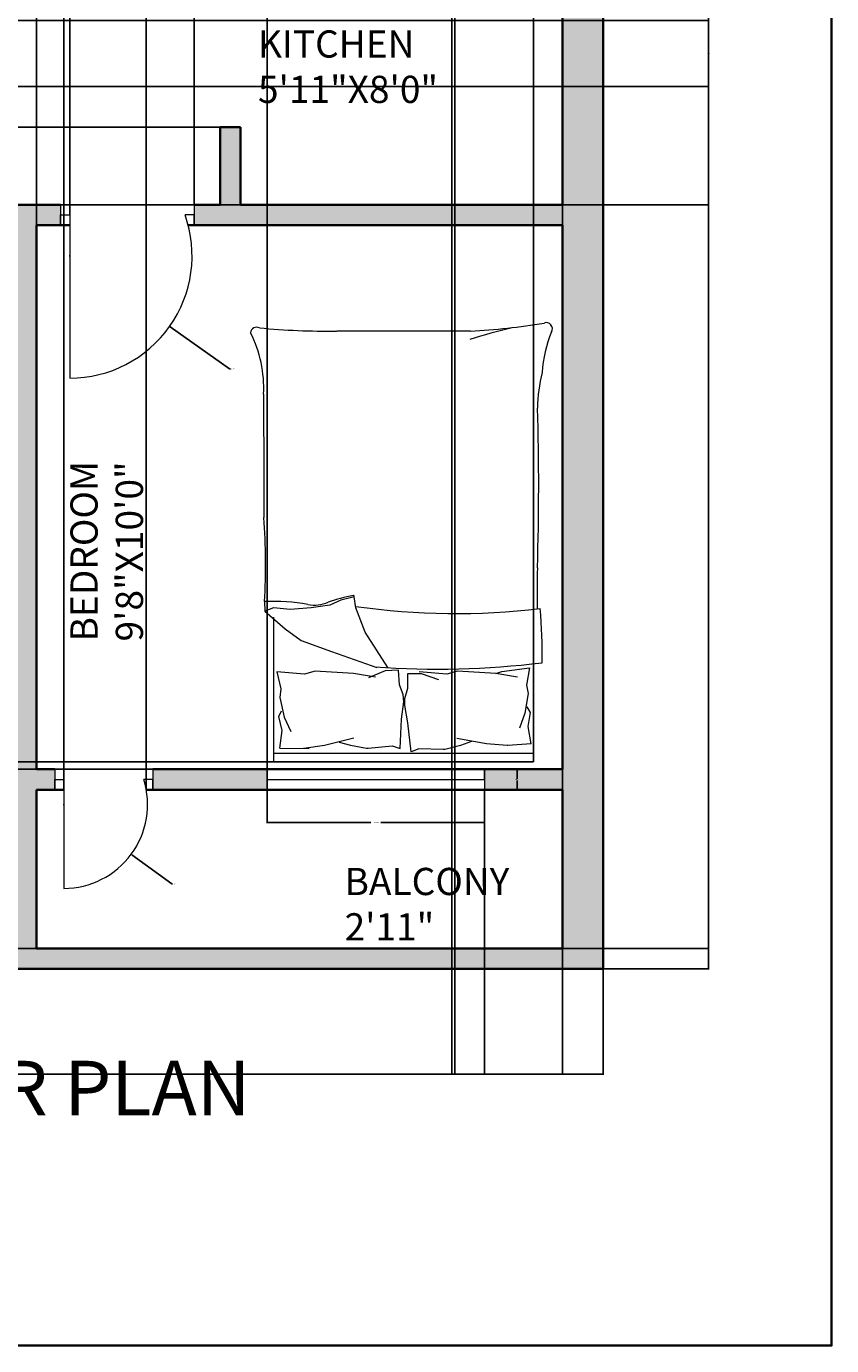
# Model space of a CAD drawing. Units: inches. Extents: x 2606 to 3027, y 1906 to 2463.
# Tile 4 of 10: x 2850 to 3027, y 1906 to 2196. Entities that reach past the tile are written whole.
import ezdxf

# ---------------------------------------------------------------- set-up
doc = ezdxf.new("R2010")
doc.units = ezdxf.units.IN
for name, color, linetype, lineweight in [('A-ANNO-DIMS', 2, 'Continuous', 18), ('A-ANNO-TEXT', 7, 'Continuous', 25), ('A-ANNO-TTLB', 7, 'Continuous', 35), ('A-AREA-IDEN', 7, 'Continuous', 18), ('A-DOOR', 3, 'Continuous', 18), ('A-FLOR-CASE', 8, 'Continuous', 18), ('A-FURN', 8, 'Continuous', 13), ('A-GLAZ', 4, 'Continuous', 18), ('A-WALL', 7, 'Continuous', 35)]:
    doc.layers.add(name, color=color, linetype=linetype, lineweight=lineweight)
doc.layers.add('A-WALL-PATT', color=251, linetype='Continuous', lineweight=13, true_color=0x636466)
doc.styles.get("Standard").update_dxf_attribs({"font": 'arial.ttf'})
doc.dimstyles.get("Standard").update_dxf_attribs({"dimtxt": 0.18, "dimasz": 0.18, "dimexe": 0.18, "dimexo": 0.0625, "dimgap": 0.09, "dimtad": 0, "dimtih": 1, "dimtoh": 1, "dimdec": 4, "dimzin": 0, "dimdsep": 46, "dimtxsty": 'Standard', "dimcen": 0.09, "dimadec": 0, "dimazin": 0, "dimtfac": 1, "dimtdec": 4, "dimtofl": 0, "dimtmove": 0, "dimatfit": 3, "dimfxl": 1, "dimtolj": 1, "dimtzin": 0, "dimarcsym": 0})

# ---------------------------------------------------------------- blocks, each defined once
blk = doc.blocks.new('BED-DOUBLE')
for p, q in [((4.17, 75.16), (4.17, 96.87)), ((4.17, 96.87), (61.46, 96.87)), ((61.46, 96.87), (61.46, 64.97)), ((4.17, 95.03), (61.46, 95.03)), ((4.67, 92.87), (9.81, 93.27)), ((9.81, 93.27), (9.93, 93.24)), ((9.93, 93.24), (14.52, 92.9)), ((17.81, 92.38), (20.24, 93.24)), ((20.24, 93.24), (23.7, 94.11)), ((23.7, 94.11), (24.09, 94.11)), ((24.09, 94.11), (29.42, 93.94)), ((29.42, 93.94), (31.15, 94.63)), ((31.15, 94.63), (31.84, 88.22)), ((33.54, 93.89), (33.25, 87.44)), ((35.31, 93.3), (33.54, 93.89)), ((40.62, 93.81), (35.31, 93.3)), ((41.01, 93.83), (40.62, 93.81)), ((44.52, 93.18), (41.01, 93.83)), ((50.25, 93.19), (43.75, 91.57)), ((47, 92.47), (44.52, 93.18)), ((54.8, 93.82), (50.25, 93.19)), ((60.08, 93.81), (53.6, 93.92)), ((53.6, 93.92), (54.8, 93.82)), ((60.08, 93.81), (59.62, 89.96)), ((4.67, 92.9), (5.36, 89.08)), ((14.52, 92.9), (21.1, 91.68)), ((59.12, 86.97), (57.7, 90.18)), ((5.36, 89.08), (4.84, 85.96)), ((6.06, 86.14), (7.27, 89.43)), ((31.84, 88.22), (32.54, 84.4)), ((33.25, 87.44), (32.79, 83.59)), ((59.62, 89.96), (60.34, 86.88)), ((4.84, 85.96), (5.54, 84.75)), ((5.36, 81.8), (6.06, 86.14)), ((32.54, 84.4), (32.54, 82.84)), ((60.08, 82.69), (59.12, 86.97)), ((60.34, 86.88), (59.72, 85.62)), ((5.71, 79.9), (5.36, 81.8)), ((32.54, 82.84), (31.84, 80.59)), ((32.79, 83.59), (32.89, 82.03)), ((32.89, 82.03), (33.72, 79.83)), ((59.85, 80.77), (60.08, 82.69)), ((5.02, 76.08), (5.71, 79.9)), ((28.9, 77.38), (25.13, 78.68)), ((31.84, 80.59), (31.84, 77.38)), ((33.72, 79.83), (33.92, 76.62)), ((60.78, 77), (59.85, 80.77)), ((11.13, 76.95), (5.02, 76.08)), ((7.65, 78.14), (12.48, 77.34)), ((12.48, 77.34), (11.13, 76.95)), ((12.48, 77.34), (20.89, 76.82)), ((20.89, 76.82), (23.24, 77.49)), ((23.24, 77.49), (29.39, 77)), ((31.84, 77.38), (28.9, 77.38)), ((33.92, 76.62), (36.87, 76.8)), ((36.28, 76.03), (41.3, 68.25)), ((36.87, 76.8), (40.55, 78.34)), ((48.73, 72.52), (38.73, 76.03)), ((39.04, 78.14), (43.87, 77.34)), ((43.87, 77.34), (52.28, 76.82)), ((52.28, 76.82), (54.63, 77.49)), ((54.63, 77.49), (60.78, 77)), ((55.41, 70.1), (48.73, 72.52)), ((58.94, 67.51), (55.41, 70.1)), ((41.3, 68.25), (43.34, 62.87)), ((63.38, 63.61), (58.94, 67.51)), ((43.34, 62.87), (43.71, 60.45)), ((43.71, 60.45), (46.68, 61.2)), ((46.68, 61.2), (49.1, 62.31)), ((49.1, 62.31), (53.18, 62.87)), ((53.18, 62.87), (57.82, 63.24)), ((57.82, 63.24), (61.54, 62.87)), ((61.54, 62.87), (63.38, 63.61)), ((63.48, 61.52), (63.38, 63.61, 4.64)), ((18.06, 1.87), (47.57, 1.87))]:
    blk.add_line(p, q)
for centre, radius, start, end in [((25.61, -121.38), 197.77, 86.0865, 96.7821), ((102.1, 72.78), 99.87, 178.7218, 185.604), ((21.29, -90.53), 154.68, 81.7845, 96.9006), ((-200.58, 59.5), 203.94, 358.4762, 1.0082), ((37.35, 95.1), 35.55, 280.6617, 289.8806), ((52.44, 54.83), 7.46, 78.6608, 113.7384), ((61.53, 104.85), 43.38, 259.8763, 272.5657), ((218.51, 53.34), 155.25, 176.9791, 183.8365), ((43.92, 60.38), 0.221, 160.2464, 271.1377), ((581.23, 36.19), 578.22, 178.22771, 181.71854), ((-5405.34, 15.56), 5469.02, 0.00217, 0.28689), ((-32.25, 19.53), 35.53, 346.0648, 358.9113), ((91.3, 14.55), 27.65, 177.4714, 206.4681), ((-25.97, 12.62), 28.25, 337.9751, 356.652), ((-20.65, 125.3), 127.63, 283.3832, 287.7053), ((1.3, 1.3), 1.31, 146.1736, 293.4781), ((25.69, -143.9), 145.97, 92.9958, 99.4091), ((49.34, -157.62), 159.5, 84.4998, 90.6351), ((65.23, 2.32), 1.32, 242.6588, 356.02)]:
    blk.add_arc(centre, radius, start, end)
blk = doc.blocks.new('WIN-48IN')
for p, q in [((0, 4.5), (0, 0)), ((48, 2.25), (48, 4.5)), ((48, 4.5), (48, 0)), ((0, 0), (0, 2.25)), ((0, 2.25), (48, 2.25))]:
    blk.add_line(p, q)
blk = doc.blocks.new('*D13')
at = {"layer": 'A-ANNO-DIMS', "color": 0, "lineweight": -2, "transparency": 16777216}
for p, q in [((2902.89, 2028.05), (2902.89, 2020.73)), ((2950.89, 2028.05), (2950.89, 2020.73)), ((2903.07, 2020.91), (2925.77, 2020.91)), ((2950.71, 2020.91), (2928.01, 2020.91))]:
    blk.add_line(p, q, dxfattribs=at)
at = {"layer": 'A-ANNO-DIMS', "color": 0, "transparency": 16777216}
for points in [[(2903.07, 2020.94), (2903.07, 2020.88), (2902.89, 2020.91)], [(2950.71, 2020.94), (2950.71, 2020.88), (2950.89, 2020.91)]]:
    blk.add_solid(points, dxfattribs=at)
at = {"layer": 'Defpoints', "color": 0, "transparency": 16777216}
for p in [(2902.89, 2028.11), (2950.89, 2028.11), (2950.89, 2020.91)]:
    blk.add_point(p, dxfattribs=at)
at = {"layer": 'A-ANNO-DIMS', "color": 0, "transparency": 16777216, "insert": (2926.89, 2020.91), "char_height": 0.18, "attachment_point": 5}
blk.add_mtext('\\A1;WINDOW 48 TYP.', dxfattribs=at)
blk = doc.blocks.new('*D14')
at = {"layer": 'A-ANNO-DIMS', "color": 0, "lineweight": -2, "transparency": 16777216}
for p, q in [((2950.95, 2032.61), (2958.27, 2032.61)), ((2958.09, 2032.43), (2958.09, 2030.54)), ((2950.95, 2028.11), (2958.27, 2028.11)), ((2958.09, 2028.29), (2958.09, 2030.18))]:
    blk.add_line(p, q, dxfattribs=at)
at = {"layer": 'A-ANNO-DIMS', "color": 0, "transparency": 16777216}
for points in [[(2958.06, 2032.43), (2958.12, 2032.43), (2958.09, 2032.61)], [(2958.06, 2028.29), (2958.12, 2028.29), (2958.09, 2028.11)]]:
    blk.add_solid(points, dxfattribs=at)
at = {"layer": 'Defpoints', "color": 0, "transparency": 16777216}
for p in [(2950.89, 2032.61), (2958.09, 2032.61), (2950.89, 2028.11)]:
    blk.add_point(p, dxfattribs=at)
at = {"layer": 'A-ANNO-DIMS', "color": 0, "transparency": 16777216, "insert": (2958.09, 2030.36), "char_height": 0.18, "attachment_point": 5}
blk.add_mtext('\\A1;5 TYP.', dxfattribs=at)
blk = doc.blocks.new('*D25')
at = {"layer": 'A-ANNO-DIMS', "color": 0, "lineweight": -2, "transparency": 16777216}
for p, q in [((2658.06, 1988.55), (2658.06, 1965.23)), ((2977.06, 1988.55), (2977.06, 1965.23)), ((2658.24, 1965.41), (2817.27, 1965.41)), ((2976.88, 1965.41), (2817.85, 1965.41))]:
    blk.add_line(p, q, dxfattribs=at)
at = {"layer": 'A-ANNO-DIMS', "color": 0, "transparency": 16777216}
for points in [[(2658.24, 1965.44), (2658.24, 1965.38), (2658.06, 1965.41)], [(2976.88, 1965.44), (2976.88, 1965.38), (2977.06, 1965.41)]]:
    blk.add_solid(points, dxfattribs=at)
at = {"layer": 'Defpoints', "color": 0, "transparency": 16777216}
for p in [(2658.06, 1988.61), (2977.06, 1988.61), (2977.06, 1965.41)]:
    blk.add_point(p, dxfattribs=at)
at = {"layer": 'A-ANNO-DIMS', "color": 0, "transparency": 16777216, "insert": (2817.56, 1965.41), "char_height": 0.18, "attachment_point": 5}
blk.add_mtext('\\A1;319', dxfattribs=at)
blk = doc.blocks.new('*D26')
at = {"layer": 'A-ANNO-DIMS', "color": 0, "lineweight": -2, "transparency": 16777216}
for p, q in [((2977.13, 2410.61), (3000.44, 2410.61)), ((3000.26, 2410.43), (3000.26, 2199.79)), ((3000.26, 1988.79), (3000.26, 2199.43)), ((2977.13, 1988.61), (3000.44, 1988.61))]:
    blk.add_line(p, q, dxfattribs=at)
at = {"layer": 'A-ANNO-DIMS', "color": 0, "transparency": 16777216}
for points in [[(3000.23, 2410.43), (3000.29, 2410.43), (3000.26, 2410.61)], [(3000.23, 1988.79), (3000.29, 1988.79), (3000.26, 1988.61)]]:
    blk.add_solid(points, dxfattribs=at)
at = {"layer": 'Defpoints', "color": 0, "transparency": 16777216}
for p in [(2977.06, 2410.61), (3000.26, 2410.61), (2977.06, 1988.61)]:
    blk.add_point(p, dxfattribs=at)
at = {"layer": 'A-ANNO-DIMS', "color": 0, "transparency": 16777216, "insert": (3000.26, 2199.61), "char_height": 0.18, "attachment_point": 5}
blk.add_mtext('\\A1;422', dxfattribs=at)
blk = doc.blocks.new('*D33')
at = {"layer": 'A-ANNO-DIMS', "color": 0, "lineweight": -2, "transparency": 16777216}
for p, q in [((2950.89, 2028.05), (2950.89, 1965.23)), ((2968.06, 2028.05), (2968.06, 1965.23)), ((2951.07, 1965.41), (2959.02, 1965.41)), ((2967.88, 1965.41), (2959.93, 1965.41))]:
    blk.add_line(p, q, dxfattribs=at)
at = {"layer": 'A-ANNO-DIMS', "color": 0, "transparency": 16777216}
for points in [[(2951.07, 1965.44), (2951.07, 1965.38), (2950.89, 1965.41)], [(2967.88, 1965.44), (2967.88, 1965.38), (2968.06, 1965.41)]]:
    blk.add_solid(points, dxfattribs=at)
at = {"layer": 'Defpoints', "color": 0, "transparency": 16777216}
for p in [(2950.89, 2028.11), (2968.06, 2028.11), (2968.06, 1965.41)]:
    blk.add_point(p, dxfattribs=at)
at = {"layer": 'A-ANNO-DIMS', "color": 0, "transparency": 16777216, "insert": (2959.48, 1965.41), "char_height": 0.18, "attachment_point": 5}
blk.add_mtext('\\A1;17.172', dxfattribs=at)
blk = doc.blocks.new('*D41')
at = {"layer": 'A-ANNO-DIMS', "color": 0, "lineweight": -2, "transparency": 16777216}
for p, q in [((2787.63, 2157.11), (3000.44, 2157.11)), ((3000.26, 2156.93), (3000.26, 2075.29)), ((3000.26, 1993.29), (3000.26, 2074.93)), ((2787.63, 1993.11), (3000.44, 1993.11))]:
    blk.add_line(p, q, dxfattribs=at)
at = {"layer": 'A-ANNO-DIMS', "color": 0, "transparency": 16777216}
for points in [[(3000.23, 2156.93), (3000.29, 2156.93), (3000.26, 2157.11)], [(3000.23, 1993.29), (3000.29, 1993.29), (3000.26, 1993.11)]]:
    blk.add_solid(points, dxfattribs=at)
at = {"layer": 'Defpoints', "color": 0, "transparency": 16777216}
for p in [(2787.56, 2157.11), (2787.56, 1993.11), (3000.26, 1993.11)]:
    blk.add_point(p, dxfattribs=at)
at = {"layer": 'A-ANNO-DIMS', "color": 0, "transparency": 16777216, "insert": (3000.26, 2075.11), "char_height": 0.18, "attachment_point": 5}
blk.add_mtext('\\A1;164', dxfattribs=at)
blk = doc.blocks.new('*D46')
at = {"layer": 'A-ANNO-DIMS', "color": 0, "lineweight": -2, "transparency": 16777216}
for p, q in [((2859.37, 2154.92), (2859.37, 2433.99)), ((2859.55, 2433.81), (2872.63, 2433.81)), ((2886.63, 2433.81), (2873.56, 2433.81)), ((2886.81, 2157.17), (2886.81, 2433.99))]:
    blk.add_line(p, q, dxfattribs=at)
at = {"layer": 'A-ANNO-DIMS', "color": 0, "transparency": 16777216}
for points in [[(2859.55, 2433.84), (2859.55, 2433.78), (2859.37, 2433.81)], [(2886.63, 2433.84), (2886.63, 2433.78), (2886.81, 2433.81)]]:
    blk.add_solid(points, dxfattribs=at)
at = {"layer": 'Defpoints', "color": 0, "transparency": 16777216}
for p in [(2886.81, 2433.81), (2886.81, 2157.11), (2859.37, 2154.86)]:
    blk.add_point(p, dxfattribs=at)
at = {"layer": 'A-ANNO-DIMS', "color": 0, "transparency": 16777216, "insert": (2873.09, 2433.81), "char_height": 0.18, "attachment_point": 5}
blk.add_mtext('\\A1;27.443', dxfattribs=at)
blk = doc.blocks.new('*D48')
at = {"layer": 'A-ANNO-DIMS', "color": 0, "lineweight": -2, "transparency": 16777216}
for p, q in [((2858.07, 2028.17), (2858.07, 2433.99)), ((2858.25, 2433.81), (2866.77, 2433.81)), ((2876.06, 2433.81), (2867.54, 2433.81)), ((2876.24, 2028.17), (2876.24, 2433.99))]:
    blk.add_line(p, q, dxfattribs=at)
at = {"layer": 'A-ANNO-DIMS', "color": 0, "transparency": 16777216}
for points in [[(2858.25, 2433.84), (2858.25, 2433.78), (2858.07, 2433.81)], [(2876.06, 2433.84), (2876.06, 2433.78), (2876.24, 2433.81)]]:
    blk.add_solid(points, dxfattribs=at)
at = {"layer": 'Defpoints', "color": 0, "transparency": 16777216}
for p in [(2876.24, 2433.81), (2858.07, 2028.11), (2876.24, 2028.11)]:
    blk.add_point(p, dxfattribs=at)
at = {"layer": 'A-ANNO-DIMS', "color": 0, "transparency": 16777216, "insert": (2867.16, 2433.81), "char_height": 0.18, "attachment_point": 5}
blk.add_mtext('\\A1;18.17', dxfattribs=at)
blk = doc.blocks.new('*D55')
at = {"layer": 'A-ANNO-DIMS', "color": 0, "lineweight": -2, "transparency": 16777216}
for p, q in [((2852.06, 2152.67), (2852.06, 2433.99)), ((2852.24, 2433.81), (2855.32, 2433.81)), ((2859.19, 2433.81), (2856.11, 2433.81)), ((2859.37, 2154.92), (2859.37, 2433.99))]:
    blk.add_line(p, q, dxfattribs=at)
at = {"layer": 'A-ANNO-DIMS', "color": 0, "transparency": 16777216}
for points in [[(2852.24, 2433.84), (2852.24, 2433.78), (2852.06, 2433.81)], [(2859.19, 2433.84), (2859.19, 2433.78), (2859.37, 2433.81)]]:
    blk.add_solid(points, dxfattribs=at)
at = {"layer": 'Defpoints', "color": 0, "transparency": 16777216}
for p in [(2859.37, 2433.81), (2859.37, 2154.86), (2852.06, 2152.61)]:
    blk.add_point(p, dxfattribs=at)
at = {"layer": 'A-ANNO-DIMS', "color": 0, "transparency": 16777216, "insert": (2855.72, 2433.81), "char_height": 0.18, "attachment_point": 5}
blk.add_mtext('\\A1;7.306', dxfattribs=at)
blk = doc.blocks.new('*D57')
at = {"layer": 'A-ANNO-DIMS', "color": 0, "lineweight": -2, "transparency": 16777216}
for p, q in [((2876.24, 2028.17), (2876.24, 2433.99)), ((2876.42, 2433.81), (2889.17, 2433.81)), ((2902.71, 2433.81), (2889.96, 2433.81)), ((2902.89, 2028.17), (2902.89, 2433.99))]:
    blk.add_line(p, q, dxfattribs=at)
at = {"layer": 'A-ANNO-DIMS', "color": 0, "transparency": 16777216}
for points in [[(2876.42, 2433.84), (2876.42, 2433.78), (2876.24, 2433.81)], [(2902.71, 2433.84), (2902.71, 2433.78), (2902.89, 2433.81)]]:
    blk.add_solid(points, dxfattribs=at)
at = {"layer": 'Defpoints', "color": 0, "transparency": 16777216}
for p in [(2902.89, 2433.81), (2876.24, 2028.11), (2902.89, 2028.11)]:
    blk.add_point(p, dxfattribs=at)
at = {"layer": 'A-ANNO-DIMS', "color": 0, "transparency": 16777216, "insert": (2889.57, 2433.81), "char_height": 0.18, "attachment_point": 5}
blk.add_mtext('\\A1;26.65', dxfattribs=at)
blk = doc.blocks.new('*D61')
at = {"layer": 'A-ANNO-DIMS', "color": 0, "lineweight": -2, "transparency": 16777216}
for p, q in [((2696.29, 2197.72), (3000.44, 2197.72)), ((3000.26, 2197.54), (3000.26, 2190.63)), ((3000.26, 2183.36), (3000.26, 2190.27)), ((2696.84, 2183.18), (3000.44, 2183.18))]:
    blk.add_line(p, q, dxfattribs=at)
at = {"layer": 'A-ANNO-DIMS', "color": 0, "transparency": 16777216}
for points in [[(3000.23, 2197.54), (3000.29, 2197.54), (3000.26, 2197.72)], [(3000.23, 2183.36), (3000.29, 2183.36), (3000.26, 2183.18)]]:
    blk.add_solid(points, dxfattribs=at)
at = {"layer": 'Defpoints', "color": 0, "transparency": 16777216}
for p in [(2696.23, 2197.72), (3000.26, 2197.72), (2696.78, 2183.18)]:
    blk.add_point(p, dxfattribs=at)
at = {"layer": 'A-ANNO-DIMS', "color": 0, "transparency": 16777216, "insert": (3000.26, 2190.45), "char_height": 0.18, "attachment_point": 5}
blk.add_mtext('\\A1;14.545', dxfattribs=at)
blk = doc.blocks.new('*D66')
at = {"layer": 'A-ANNO-DIMS', "color": 0, "lineweight": -2, "transparency": 16777216}
for p, q in [((2968.06, 2253.05), (2968.06, 1965.23)), ((2944.33, 2234.06), (2944.33, 1965.23)), ((2944.51, 1965.41), (2955.8, 1965.41)), ((2967.88, 1965.41), (2956.59, 1965.41))]:
    blk.add_line(p, q, dxfattribs=at)
at = {"layer": 'A-ANNO-DIMS', "color": 0, "transparency": 16777216}
for points in [[(2944.51, 1965.44), (2944.51, 1965.38), (2944.33, 1965.41)], [(2967.88, 1965.44), (2967.88, 1965.38), (2968.06, 1965.41)]]:
    blk.add_solid(points, dxfattribs=at)
at = {"layer": 'Defpoints', "color": 0, "transparency": 16777216}
for p in [(2968.06, 2253.11), (2944.33, 2234.12), (2968.06, 1965.41)]:
    blk.add_point(p, dxfattribs=at)
at = {"layer": 'A-ANNO-DIMS', "color": 0, "transparency": 16777216, "insert": (2956.2, 1965.41), "char_height": 0.18, "attachment_point": 5}
blk.add_mtext('\\A1;23.73', dxfattribs=at)
blk = doc.blocks.new('*D68')
at = {"layer": 'A-ANNO-DIMS', "color": 0, "lineweight": -2, "transparency": 16777216}
for p, q in [((2897, 2215.13), (2634.68, 2215.13)), ((2634.86, 2214.95), (2634.86, 2194.85)), ((2634.86, 2174.38), (2634.86, 2194.48)), ((2897, 2174.2), (2634.68, 2174.2))]:
    blk.add_line(p, q, dxfattribs=at)
at = {"layer": 'A-ANNO-DIMS', "color": 0, "transparency": 16777216}
for points in [[(2634.83, 2214.95), (2634.89, 2214.95), (2634.86, 2215.13)], [(2634.83, 2174.38), (2634.89, 2174.38), (2634.86, 2174.2)]]:
    blk.add_solid(points, dxfattribs=at)
at = {"layer": 'Defpoints', "color": 0, "transparency": 16777216}
for p in [(2897.06, 2215.13), (2634.86, 2174.2), (2897.06, 2174.2)]:
    blk.add_point(p, dxfattribs=at)
at = {"layer": 'A-ANNO-DIMS', "color": 0, "transparency": 16777216, "insert": (2634.86, 2194.66), "char_height": 0.18, "attachment_point": 5}
blk.add_mtext('\\A1;40.94', dxfattribs=at)
blk = doc.blocks.new('*D69')
at = {"layer": 'A-ANNO-DIMS', "color": 0, "lineweight": -2, "transparency": 16777216}
for p, q in [((2897, 2174.2), (2634.68, 2174.2)), ((2634.86, 2174.02), (2634.86, 2165.84)), ((2634.86, 2157.29), (2634.86, 2165.47)), ((2897, 2157.11), (2634.68, 2157.11))]:
    blk.add_line(p, q, dxfattribs=at)
at = {"layer": 'A-ANNO-DIMS', "color": 0, "transparency": 16777216}
for points in [[(2634.83, 2174.02), (2634.89, 2174.02), (2634.86, 2174.2)], [(2634.83, 2157.29), (2634.89, 2157.29), (2634.86, 2157.11)]]:
    blk.add_solid(points, dxfattribs=at)
at = {"layer": 'Defpoints', "color": 0, "transparency": 16777216}
for p in [(2897.06, 2174.2), (2634.86, 2157.11), (2897.06, 2157.11)]:
    blk.add_point(p, dxfattribs=at)
at = {"layer": 'A-ANNO-DIMS', "color": 0, "transparency": 16777216, "insert": (2634.86, 2165.65), "char_height": 0.18, "attachment_point": 5}
blk.add_mtext('\\A1;17.087', dxfattribs=at)
blk = doc.blocks.new('*D75')
at = {"layer": 'A-ANNO-DIMS', "color": 0, "lineweight": -2, "transparency": 16777216}
for p, q in [((2968.06, 2401.55), (2968.06, 1965.23)), ((2943.67, 2399.33), (2943.67, 1965.23)), ((2943.85, 1965.41), (2955.4, 1965.41)), ((2967.88, 1965.41), (2956.33, 1965.41))]:
    blk.add_line(p, q, dxfattribs=at)
at = {"layer": 'A-ANNO-DIMS', "color": 0, "transparency": 16777216}
for points in [[(2943.85, 1965.44), (2943.85, 1965.38), (2943.67, 1965.41)], [(2967.88, 1965.44), (2967.88, 1965.38), (2968.06, 1965.41)]]:
    blk.add_solid(points, dxfattribs=at)
at = {"layer": 'Defpoints', "color": 0, "transparency": 16777216}
for p in [(2968.06, 2401.61), (2943.67, 2399.4), (2968.06, 1965.41)]:
    blk.add_point(p, dxfattribs=at)
at = {"layer": 'A-ANNO-DIMS', "color": 0, "transparency": 16777216, "insert": (2955.86, 1965.41), "char_height": 0.18, "attachment_point": 5}
blk.add_mtext('\\A1;24.397', dxfattribs=at)
blk = doc.blocks.new('*D77')
at = {"layer": 'A-ANNO-DIMS', "color": 0, "lineweight": -2, "transparency": 16777216}
for p, q in [((2961.66, 2034.29), (2961.66, 2433.99)), ((2961.84, 2433.81), (2964.47, 2433.81)), ((2967.88, 2433.81), (2965.26, 2433.81)), ((2968.06, 2032.67), (2968.06, 2433.99))]:
    blk.add_line(p, q, dxfattribs=at)
at = {"layer": 'A-ANNO-DIMS', "color": 0, "transparency": 16777216}
for points in [[(2961.84, 2433.84), (2961.84, 2433.78), (2961.66, 2433.81)], [(2967.88, 2433.84), (2967.88, 2433.78), (2968.06, 2433.81)]]:
    blk.add_solid(points, dxfattribs=at)
at = {"layer": 'Defpoints', "color": 0, "transparency": 16777216}
for p in [(2968.06, 2433.81), (2961.66, 2034.23), (2968.06, 2032.61)]:
    blk.add_point(p, dxfattribs=at)
at = {"layer": 'A-ANNO-DIMS', "color": 0, "transparency": 16777216, "insert": (2964.86, 2433.81), "char_height": 0.18, "attachment_point": 5}
blk.add_mtext('\\A1;6.402', dxfattribs=at)
blk = doc.blocks.new('*D81')
at = {"layer": 'A-ANNO-DIMS', "color": 0, "lineweight": -2, "transparency": 16777216}
for p, q in [((2961.6, 2034.23), (2634.68, 2034.23)), ((2634.86, 2034.05), (2634.86, 2033.6)), ((2950.83, 2032.61), (2634.68, 2032.61)), ((2634.86, 2032.79), (2634.86, 2033.24))]:
    blk.add_line(p, q, dxfattribs=at)
at = {"layer": 'A-ANNO-DIMS', "color": 0, "transparency": 16777216}
for points in [[(2634.83, 2034.05), (2634.89, 2034.05), (2634.86, 2034.23)], [(2634.83, 2032.79), (2634.89, 2032.79), (2634.86, 2032.61)]]:
    blk.add_solid(points, dxfattribs=at)
at = {"layer": 'Defpoints', "color": 0, "transparency": 16777216}
for p in [(2961.66, 2034.23), (2634.86, 2032.61), (2950.89, 2032.61)]:
    blk.add_point(p, dxfattribs=at)
at = {"layer": 'A-ANNO-DIMS', "color": 0, "transparency": 16777216, "insert": (2634.86, 2033.42), "char_height": 0.18, "attachment_point": 5}
blk.add_mtext('\\A1;1.62', dxfattribs=at)
blk = doc.blocks.new('*D87')
at = {"layer": 'A-ANNO-DIMS', "color": 0, "lineweight": -2, "transparency": 16777216}
for p, q in [((2859.28, 2145.85), (2859.46, 2145.85)), ((2859.37, 2145.76), (2859.37, 2145.94)), ((2894.64, 2120.93), (2881.56, 2130.17)), ((2894.82, 2120.93), (2894.64, 2120.93))]:
    blk.add_line(p, q, dxfattribs=at)
at = {"layer": 'A-ANNO-DIMS', "color": 0, "transparency": 16777216}
blk.add_solid([(2881.58, 2130.19), (2881.54, 2130.14), (2881.41, 2130.27)], dxfattribs=at)
at = {"layer": 'Defpoints', "color": 0, "transparency": 16777216}
for p in [(2859.37, 2145.85), (2881.41, 2130.27)]:
    blk.add_point(p, dxfattribs=at)
at = {"layer": 'A-ANNO-DIMS', "color": 0, "transparency": 16777216, "insert": (2895.3, 2120.93), "char_height": 0.18, "attachment_point": 5}
blk.add_mtext('\\A1;R26.99', dxfattribs=at)
blk = doc.blocks.new('*D89')
at = {"layer": 'A-ANNO-DIMS', "color": 0, "lineweight": -2, "transparency": 16777216}
for p, q in [((2857.98, 2024.82), (2858.16, 2024.82)), ((2858.07, 2024.73), (2858.07, 2024.91)), ((2881.89, 2007.34), (2873.1, 2013.79)), ((2882.07, 2007.34), (2881.89, 2007.34))]:
    blk.add_line(p, q, dxfattribs=at)
at = {"layer": 'A-ANNO-DIMS', "color": 0, "transparency": 16777216}
blk.add_solid([(2873.12, 2013.82), (2873.09, 2013.77), (2872.96, 2013.9)], dxfattribs=at)
at = {"layer": 'Defpoints', "color": 0, "transparency": 16777216}
for p in [(2858.07, 2024.82), (2872.96, 2013.9)]:
    blk.add_point(p, dxfattribs=at)
at = {"layer": 'A-ANNO-DIMS', "color": 0, "transparency": 16777216, "insert": (2882.62, 2007.34), "char_height": 0.18, "attachment_point": 5}
blk.add_mtext('\\A1;R18.464', dxfattribs=at)

msp = doc.modelspace()

# ---------------------------------------------------------------- hatches: boundary and pattern name
at = {"layer": 'A-WALL-PATT'}
h = msp.add_hatch(color=256, dxfattribs=at)
h.dxf.hatch_style = 1
h.paths.add_polyline_path([(2667.063, 2401.6097), (2691.9697, 2401.6097), (2691.9697, 2406.1097), (2691.9697, 2410.6097), (2658.063, 2410.6097), (2658.063, 2238.7051), (2667.063, 2238.7051)])
h.paths.add_polyline_path([(2804.9965, 2406.1097), (2804.9965, 2410.6097), (2751.9697, 2410.6097), (2751.9697, 2401.6097), (2783.063, 2401.6097), (2783.063, 2257.6097), (2778.6739, 2257.6097), (2778.6739, 2253.1097), (2792.3386, 2253.1097), (2792.3386, 2255.3597), (2792.3386, 2257.6097), (2787.563, 2257.6097), (2787.563, 2327.1097), (2847.563, 2327.1097), (2847.563, 2331.6097), (2787.563, 2331.6097), (2787.563, 2401.6097), (2804.9965, 2401.6097)])
h.paths.add_polyline_path([(2889.6183, 2406.1097), (2889.6183, 2410.6097), (2828.9965, 2410.6097), (2828.9965, 2401.6097), (2831.8174, 2401.6097), (2847.563, 2401.6097), (2847.563, 2357.8311), (2849.813, 2357.8311), (2852.063, 2357.8311), (2852.063, 2401.6097), (2889.6183, 2401.6097)])
h.paths.add_polyline_path([(2977.063, 2410.6097), (2949.6183, 2410.6097), (2949.6183, 2401.6097), (2968.063, 2401.6097), (2968.063, 2157.1097), (2897.063, 2157.1097), (2897.063, 2174.1966), (2892.563, 2174.1966), (2892.563, 2157.1097), (2886.8122, 2157.1097), (2886.8122, 2152.6097), (2968.063, 2152.6097), (2968.063, 2032.6097), (2950.8911, 2032.6097), (2950.8911, 2028.1097), (2968.063, 2028.1097), (2968.063, 1993.1097), (2852.063, 1993.1097), (2852.063, 2028.1097), (2856.0743, 2028.1097), (2856.0743, 2030.3597), (2856.0743, 2032.6097), (2852.063, 2032.6097), (2852.063, 2152.6097), (2857.369, 2152.6097), (2857.369, 2154.8597), (2857.369, 2157.1097), (2847.563, 2157.1097), (2847.563, 2152.6097), (2847.563, 1993.1097), (2837.0415, 1993.1097), (2837.0415, 1988.6097), (2977.063, 1988.6097)])
h.paths.add_polyline_path([(2968.063, 2257.6097), (2886.9679, 2257.6097), (2886.9679, 2253.1097), (2892.563, 2253.1097), (2892.563, 2215.1332), (2897.063, 2215.1332), (2897.063, 2253.1097), (2968.063, 2253.1097)], flags=17)
h.paths.add_polyline_path([(2856.057, 2255.3597), (2856.057, 2257.6097), (2852.063, 2257.6097), (2852.063, 2336.7476), (2849.813, 2336.7476), (2847.563, 2336.7476), (2847.563, 2331.6097), (2847.563, 2327.1097), (2847.563, 2257.6097), (2813.482, 2257.6097), (2813.482, 2253.1097), (2856.057, 2253.1097)])
h.paths.add_polyline_path([(2748.8874, 2255.3597), (2748.8874, 2257.6097), (2667.063, 2257.6097), (2667.063, 2253.1097), (2748.8874, 2253.1097)])
h.paths.add_polyline_path([(2667.063, 2152.6097), (2744.8238, 2152.6097), (2744.8238, 2154.8597), (2744.8238, 2157.1097), (2667.063, 2157.1097), (2667.063, 2178.7051), (2658.063, 2178.7051), (2658.063, 1988.6097), (2801.0415, 1988.6097), (2801.0415, 1990.8597), (2801.0415, 1993.1097), (2787.563, 1993.1097), (2787.563, 2157.1097), (2777.1295, 2157.1097), (2777.1295, 2152.6097), (2783.063, 2152.6097), (2783.063, 2032.6097), (2778.4484, 2032.6097), (2778.4484, 2028.1097), (2783.063, 2028.1097), (2783.063, 1993.1097), (2667.063, 1993.1097), (2667.063, 2028.1097), (2680.1652, 2028.1097), (2680.1652, 2030.3597), (2680.1652, 2032.6097), (2667.063, 2032.6097)])
h.paths.add_polyline_path([(2755.4074, 2032.6097), (2728.1652, 2032.6097), (2728.1652, 2028.1097), (2755.4074, 2028.1097), (2755.4074, 2030.3597)], flags=17)
h.paths.add_polyline_path([(2902.8911, 2030.3597), (2902.8911, 2032.6097), (2877.6885, 2032.6097), (2877.6885, 2028.1097), (2902.8911, 2028.1097)], flags=17)
h.paths.add_polyline_path([(2810.2211, 2267.221), (2851.2716, 2267.221), (2851.2716, 2289.6098), (2810.2211, 2289.6098)], flags=9)

# ---------------------------------------------------------------- linework, layer by layer
at = {"layer": 'A-ANNO-TTLB'}
msp.add_lwpolyline([(2605.9227, 2462.7868), (3027.4339, 2462.7868), (3027.4339, 1905.5336), (2605.9227, 1905.5336)], close=True, dxfattribs=at)
at = {"layer": 'A-DOOR'}
for p, q in [((2857.369, 2157.1097), (2857.369, 2152.6097)), ((2886.8122, 2157.1097), (2886.8122, 2152.6097)), ((2857.369, 2152.6097), (2857.369, 2154.8597)), ((2857.369, 2154.8597), (2859.369, 2154.8597)), ((2859.369, 2154.8597), (2859.369, 2118.8597)), ((2886.8122, 2154.8597), (2884.8122, 2154.8597)), ((2886.8122, 2152.6097), (2886.8122, 2154.8597)), ((2856.0743, 2032.6097), (2856.0743, 2028.1097)), ((2877.6885, 2032.6097), (2877.6885, 2032.6097)), ((2877.6885, 2032.6097), (2877.6885, 2028.1097)), ((2856.0743, 2028.1097), (2856.0743, 2030.3597)), ((2856.0743, 2030.3597), (2858.0743, 2030.3597)), ((2858.0743, 2030.3597), (2858.0743, 2006.3597)), ((2877.6885, 2030.3597), (2875.6885, 2030.3597)), ((2877.6885, 2028.1097), (2877.6885, 2030.3597))]:
    msp.add_line(p, q, dxfattribs=at)
for centre, radius, end in [((2859.369, 2145.8508), 26.9911, 19.497898), ((2858.0743, 2024.8235), 18.4638, 17.448221)]:
    msp.add_arc(centre, radius, 270, end, dxfattribs=at)
at = {"layer": 'A-FLOR-CASE'}
msp.add_line((2944.3333, 2234.1214), (2944.3333, 2157.1097), dxfattribs=at)
at = {"layer": 'A-WALL'}
for p, q in [((2977.063, 2410.6097), (2977.063, 1988.6097)), ((2968.063, 2401.6097), (2968.063, 2157.1097)), ((2892.563, 2174.1966), (2897.063, 2174.1966)), ((2892.563, 2174.1966), (2892.563, 2157.1097)), ((2897.063, 2157.1097), (2897.063, 2174.1966)), ((2847.563, 2157.1097), (2857.369, 2157.1097)), ((2847.563, 2157.1097), (2857.369, 2157.1097)), ((2886.8122, 2157.1097), (2892.563, 2157.1097)), ((2968.063, 2157.1097), (2897.063, 2157.1097)), ((2897.063, 2157.1097), (2968.063, 2157.1097)), ((2852.063, 2152.6097), (2852.063, 2032.6097)), ((2852.063, 2152.6097), (2859.369, 2152.6097)), ((2885.5001, 2152.6097), (2968.063, 2152.6097)), ((2968.063, 2152.6097), (2968.063, 2032.6097)), ((2852.063, 2032.6097), (2856.0743, 2032.6097)), ((2877.6885, 2032.6097), (2968.063, 2032.6097)), ((2852.063, 2028.1097), (2858.0743, 2028.1097)), ((2852.063, 2028.1097), (2852.063, 1993.1097)), ((2876.2433, 2028.1097), (2968.063, 2028.1097)), ((2968.063, 2028.1097), (2968.063, 1993.1097)), ((2852.063, 1993.1097), (2968.063, 1993.1097)), ((2658.063, 1988.6097), (2977.063, 1988.6097))]:
    msp.add_line(p, q, dxfattribs=at)

# ---------------------------------------------------------------- block references
at = {"layer": 'A-FURN', "rotation": 180}
msp.add_blockref('BED-DOUBLE', (2965.8274, 2131.1025), dxfattribs=at)
at = {"layer": 'A-GLAZ'}
msp.add_blockref('WIN-48IN', (2902.891, 2028.11), dxfattribs=at)

# ---------------------------------------------------------------- texts
at = {"layer": 'A-ANNO-TEXT', "insert": (2754.4391, 1968.3416), "char_height": 12, "attachment_point": 1}
msp.add_mtext_dynamic_manual_height_columns('FIRST FLOOR PLAN', width=233.480418, gutter_width=12.5, heights=[0], dxfattribs=at)
at = {"layer": 'A-AREA-IDEN', "char_height": 6, "attachment_point": 1}
for s, width, insert in [('KITCHEN\\P5\'11"X8\'0"', 83.924952, (2900.9027, 2195.5474)), ('BALCONY\\P2\'11"', 32.965259, (2919.9963, 2010.8806))]:
    msp.add_mtext_dynamic_manual_height_columns(s, width=width, gutter_width=12.5, heights=[0], dxfattribs=dict(at, insert=insert))
at = {"layer": 'A-AREA-IDEN', "insert": (2859.5331, 2060.7956), "char_height": 6, "attachment_point": 1, "rotation": 90}
msp.add_mtext_dynamic_manual_height_columns('BEDROOM\\P9\'8"X10\'0"', width=82.620136, gutter_width=12.5, heights=[0], dxfattribs=at)

# ---------------------------------------------------------------- dimensions: what is measured, and where the dimension line sits
at = {"layer": 'A-ANNO-DIMS'}
for base, p1, p2, override, picture, middle in [((2859.369, 2433.8097), (2852.063, 2152.6097), (2859.369, 2154.8597), {"dimdec": 3, "dimlfac": 1, "dimrnd": 0, "dimzin": 0, "dimdsep": 46, "dimlunit": 2}, '*D55', (2855.716, 2433.8097)), ((2876.2433, 2433.8097), (2858.0743, 2028.1097), (2876.2433, 2028.1097), {"dimdec": 2, "dimlfac": 1, "dimrnd": 0, "dimzin": 0, "dimdsep": 46, "dimlunit": 2}, '*D48', (2867.1588, 2433.8097)), ((2886.8122, 2433.8097), (2859.369, 2154.8597), (2886.8122, 2157.1097), {"dimdec": 3, "dimlfac": 1, "dimrnd": 0, "dimzin": 0, "dimdsep": 46, "dimlunit": 2}, '*D46', (2873.0906, 2433.8097)), ((2902.8911, 2433.8097), (2876.2433, 2028.1097), (2902.8911, 2028.1097), {"dimdec": 2, "dimlfac": 1, "dimrnd": 0, "dimzin": 0, "dimdsep": 46, "dimlunit": 2}, '*D57', (2889.5672, 2433.8097)), ((2968.063, 2433.8097), (2961.6611, 2034.2301), (2968.063, 2032.6097), {"dimdec": 3, "dimlfac": 1, "dimrnd": 0, "dimzin": 0, "dimdsep": 46, "dimlunit": 2}, '*D77', (2964.8621, 2433.8097)), ((2968.063, 1965.4097), (2943.6661, 2399.3963), (2968.063, 2401.6097), {"dimdec": 3, "dimlfac": 1, "dimrnd": 0, "dimzin": 0, "dimdsep": 46, "dimlunit": 2}, '*D75', (2955.8645, 1965.4097)), ((2968.063, 1965.4097), (2944.3333, 2234.1214), (2968.063, 2253.1097), {"dimdec": 2, "dimlfac": 1, "dimrnd": 0, "dimzin": 0, "dimdsep": 46, "dimlunit": 2}, '*D66', (2956.1982, 1965.4097)), ((2968.063, 1965.4097), (2950.8911, 2028.1097), (2968.063, 2028.1097), {"dimdec": 3, "dimlfac": 1, "dimrnd": 0, "dimzin": 0, "dimdsep": 46, "dimlunit": 2}, '*D33', (2959.4771, 1965.4097)), ((2977.063, 1965.4097), (2658.063, 1988.6097), (2977.063, 1988.6097), {"dimdec": 0, "dimlfac": 1, "dimrnd": 0, "dimzin": 0, "dimdsep": 46, "dimlunit": 2}, '*D25', (2817.563, 1965.4097))]:
    dim = msp.add_linear_dim(base=base, p1=p1, p2=p2, dimstyle='Standard', override=override, dxfattribs=at)
    dim.commit()
    dim.dimension.update_dxf_attribs({"geometry": picture, "text_midpoint": middle})
for base, p1, p2, override, picture, middle in [((3000.263, 2410.6097), (2977.063, 1988.6097), (2977.063, 2410.6097), {"dimdec": 0, "dimlfac": 1, "dimrnd": 0, "dimzin": 0, "dimdsep": 46, "dimlunit": 2}, '*D26', (3000.263, 2199.6097)), ((2634.863, 2174.1966), (2897.063, 2215.1332), (2897.063, 2174.1966), {"dimdec": 2, "dimlfac": 1, "dimrnd": 0, "dimzin": 0, "dimdsep": 46, "dimlunit": 2}, '*D68', (2634.863, 2194.6649)), ((3000.263, 2197.7249), (2696.782, 2183.1802), (2696.232, 2197.7249), {"dimdec": 3, "dimlfac": 1, "dimrnd": 0, "dimzin": 0, "dimdsep": 46, "dimlunit": 2}, '*D61', (3000.263, 2190.4526)), ((2634.863, 2157.1097), (2897.063, 2174.1966), (2897.063, 2157.1097), {"dimdec": 3, "dimlfac": 1, "dimrnd": 0, "dimzin": 0, "dimdsep": 46, "dimlunit": 2}, '*D69', (2634.863, 2165.6532)), ((3000.263, 1993.1097), (2787.563, 2157.1097), (2787.563, 1993.1097), {"dimdec": 0, "dimlfac": 1, "dimrnd": 0, "dimzin": 0, "dimdsep": 46, "dimlunit": 2}, '*D41', (3000.263, 2075.1097)), ((2634.863, 2032.6097), (2961.6611, 2034.2301), (2950.8911, 2032.6097), {"dimdec": 2, "dimlfac": 1, "dimrnd": 0, "dimzin": 0, "dimdsep": 46, "dimlunit": 2}, '*D81', (2634.863, 2033.4199))]:
    dim = msp.add_linear_dim(base=base, p1=p1, p2=p2, angle=90, dimstyle='Standard', override=override, dxfattribs=at)
    dim.commit()
    dim.dimension.update_dxf_attribs({"geometry": picture, "text_midpoint": middle})
for center, mpoint, override, picture, middle in [((2859.369, 2145.8508), (2881.411, 2130.273), {"dimdec": 2, "dimlfac": 1, "dimrnd": 0, "dimzin": 0, "dimdsep": 46, "dimlunit": 2}, '*D87', (2895.2963, 2120.9263)), ((2858.0743, 2024.8235), (2872.9593, 2013.8988), {"dimdec": 3, "dimlfac": 1, "dimrnd": 0, "dimzin": 0, "dimdsep": 46, "dimlunit": 2}, '*D89', (2882.6197, 2007.344))]:
    dim = msp.add_radius_dim(center=center, mpoint=mpoint, dimstyle='Standard', override=override, dxfattribs=at)
    dim.commit()
    dim.dimension.update_dxf_attribs({"geometry": picture, "text_midpoint": middle, "dimtype": 164})
dim = msp.add_linear_dim(base=(2958.091106974, 2032.6096955265), p1=(2950.891106974, 2028.1096955265), p2=(2950.891106974, 2032.6096955265), angle=90, text='<> TYP.', dimstyle='Standard', override={"dimdec": 0, "dimlfac": 1, "dimrnd": 0, "dimzin": 0, "dimdsep": 46, "dimlunit": 2}, dxfattribs=at)
dim.commit()
dim.dimension.update_dxf_attribs({"geometry": '*D14', "text_midpoint": (2958.091106974, 2030.3596955265)})
dim = msp.add_linear_dim(base=(2950.8911, 2020.9097), p1=(2902.8911, 2028.1097), p2=(2950.8911, 2028.1097), text='WINDOW <> TYP.', dimstyle='Standard', override={"dimdec": 0, "dimlfac": 1, "dimrnd": 0, "dimzin": 0, "dimdsep": 46, "dimlunit": 2}, dxfattribs=at)
dim.commit()
dim.dimension.update_dxf_attribs({"geometry": '*D13', "text_midpoint": (2926.8911, 2020.9097)})

doc.saveas('drawing.dxf')
